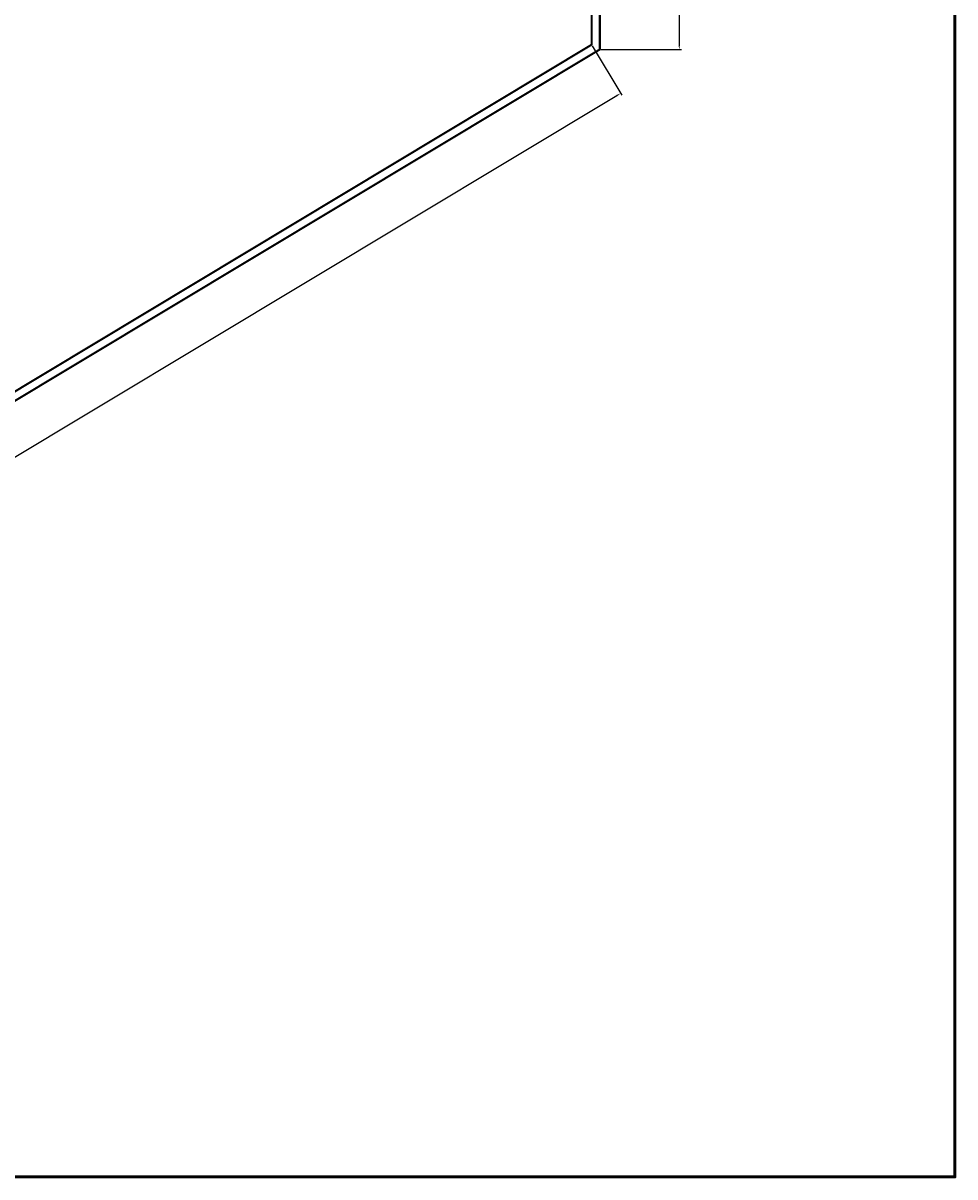
# Model space of a CAD drawing. Units: millimetres. Extents: x 2134 to 3363, y 1052 to 3233.
# Tile 4 of 11: x 2854 to 3363, y 1152 to 1782. Entities that reach past the tile are written whole.
import ezdxf

# ---------------------------------------------------------------- set-up
doc = ezdxf.new("R2010")
doc.units = ezdxf.units.MM
for name, color, linetype, lineweight in [('A-ANNO-DIMS', 2, 'Continuous', 18), ('A-ANNO-TTLB', 7, 'Continuous', 50), ('C-PROP', 6, 'Continuous', 35)]:
    doc.layers.add(name, color=color, linetype=linetype, lineweight=lineweight)
doc.styles.get("Standard").update_dxf_attribs({"font": 'arial.ttf'})
doc.dimstyles.new('ISO-25', dxfattribs={"dimtxt": 2.5, "dimasz": 2.5, "dimexe": 1.25, "dimexo": 0.625, "dimtad": 1, "dimtxsty": 'Standard', "dimcen": 2.5, "dimadec": 0, "dimazin": 0, "dimtfac": 1, "dimtmove": 0, "dimatfit": 3, "dimfxl": 1, "dimarcsym": 0})

# ---------------------------------------------------------------- blocks, each defined once
blk = doc.blocks.new('*D9')
at = {"layer": 'A-ANNO-DIMS', "color": 0, "lineweight": -2, "transparency": 16777216}
for p, q in [((3169.46, 3063.82), (3213.48, 3063.82)), ((3212.23, 3061.32), (3212.23, 1770.32)), ((3169.46, 1767.82), (3213.48, 1767.82))]:
    blk.add_line(p, q, dxfattribs=at)
at = {"layer": 'A-ANNO-DIMS', "color": 0, "transparency": 16777216}
for points in [[(3211.81, 3061.32), (3212.65, 3061.32), (3212.23, 3063.82)], [(3211.81, 1770.32), (3212.65, 1770.32), (3212.23, 1767.82)]]:
    blk.add_solid(points, dxfattribs=at)
at = {"layer": 'Defpoints', "color": 0, "transparency": 16777216}
for p in [(3168.84, 3063.82), (3168.84, 1767.82), (3212.23, 1767.82)]:
    blk.add_point(p, dxfattribs=at)
at = {"layer": 'A-ANNO-DIMS', "color": 0, "transparency": 16777216, "insert": (3210.33, 2415.82), "char_height": 2.5, "attachment_point": 5, "rotation": 90}
blk.add_mtext('1296', dxfattribs=at)
blk = doc.blocks.new('*D10')
at = {"layer": 'A-ANNO-DIMS', "color": 0, "lineweight": -2, "transparency": 16777216}
for p, q in [((3164.66, 1769.83), (3180.9, 1742.8)), ((3178.12, 1742.58), (2221.66, 1167.89)), ((2203.92, 1192.56), (2220.16, 1165.53))]:
    blk.add_line(p, q, dxfattribs=at)
at = {"layer": 'A-ANNO-DIMS', "color": 0, "transparency": 16777216}
for points in [[(3177.9, 1742.94), (3178.33, 1742.23), (3180.26, 1743.87)], [(2221.44, 1168.24), (2221.87, 1167.53), (2219.52, 1166.6)]]:
    blk.add_solid(points, dxfattribs=at)
at = {"layer": 'Defpoints', "color": 0, "transparency": 16777216}
for p in [(3164.34, 1770.37), (2203.6, 1193.09), (2219.52, 1166.6)]:
    blk.add_point(p, dxfattribs=at)
at = {"layer": 'A-ANNO-DIMS', "color": 0, "transparency": 16777216, "insert": (2674.71, 1442.59), "char_height": 2.5, "attachment_point": 5, "rotation": 31}
blk.add_mtext('1120,83', dxfattribs=at)

msp = doc.modelspace()

# ---------------------------------------------------------------- linework, layer by layer
at = {"layer": 'A-ANNO-TTLB', "ltscale": 0.5}
msp.add_lwpolyline([(2134.34, 3233.23), (3362.77, 3233.23), (3362.77, 1152.237), (2134.34, 1152.237)], close=True, dxfattribs=at)
at = {"layer": 'C-PROP'}
for p, q in [((3168.839, 3063.82), (3168.839, 1767.82)), ((3164.339, 3059.32), (3164.339, 1770.366)), ((3168.839, 1767.82), (3168.839, 2232.82)), ((3164.339, 1770.366), (2203.596, 1193.093)), ((3168.839, 1767.82), (2197.066, 1183.92))]:
    msp.add_line(p, q, dxfattribs=at)

# ---------------------------------------------------------------- dimensions: what is measured, and where the dimension line sits
at = {"layer": 'A-ANNO-DIMS'}
dim = msp.add_linear_dim(base=(3212.229, 1767.82), p1=(3168.839, 3063.82), p2=(3168.839, 1767.82), angle=90, dimstyle='ISO-25', override={"dimclrd": 0, "dimclre": 0, "dimclrt": 0}, dxfattribs=at)
dim.commit()
dim.dimension.update_dxf_attribs({"geometry": '*D9', "text_midpoint": (3210.327, 2415.82)})
dim = msp.add_linear_dim(base=(2219.5153, 1166.599), p1=(3164.339, 1770.3661), p2=(2203.5959, 1193.0934), angle=211, dimstyle='ISO-25', override={"dimclrd": 0, "dimclre": 0, "dimclrt": 0}, dxfattribs=at)
dim.commit()
dim.dimension.update_dxf_attribs({"geometry": '*D10', "text_midpoint": (2675.8085, 1440.7677), "dimtype": 161})

doc.saveas('drawing.dxf')
